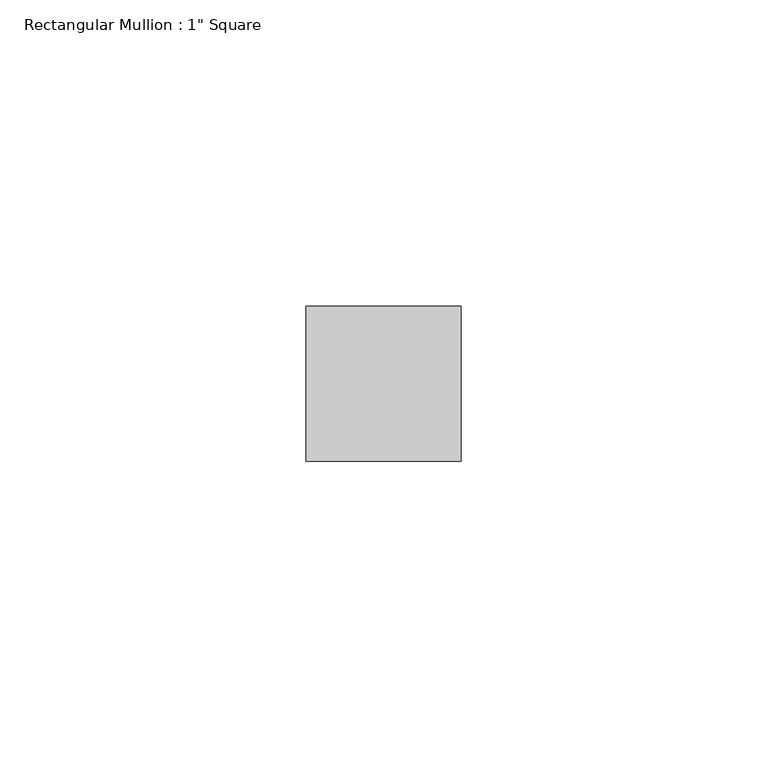
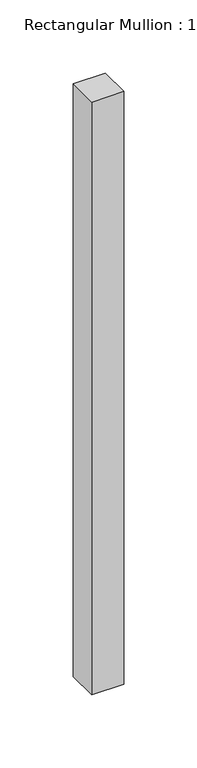
"""IFC4 building model written with IfcOpenShell, lengths in millimetres: member geometry."""

from ifc_helpers import new_model, si_unit, frame, origin, place, context, project, spatial, polyline, outline, extrude, source, transform, mapped, element, save


def member_84e80635(model_context):
    return source(origin(), model_context, "Body", "SweptSolid", [
        extrude(outline(polyline([(0.0, 12.7), (0.0, -12.7), (-25.4, -12.7), (-25.4, 12.7), (0.0, 12.7)])), frame((0.0, 0.0, -495.6398623), z_axis=(0.0, 0.0, 1.0), x_axis=(1.0, 0.0, 0.0)), (0.0, 0.0, 1.0), 495.6398623),
    ])


if __name__ == "__main__":
    model = new_model("IFC4")
    model_context = context("Model", 3, world=origin())
    ifc_project = project(units=[si_unit("LENGTHUNIT", "METRE", prefix="MILLI")], contexts=[model_context])
    site = spatial("IfcSite", under=ifc_project)
    building = spatial("IfcBuilding", under=site)
    placement = place(None, origin())
    member_shape = member_84e80635(model_context)
    element("IfcMember", 1, ObjectType="Rectangular Mullion : 1\" Square", at=placement, inside=building, context=model_context, shape_type="MappedRepresentation", body=[
        mapped(member_shape, transform((0.0, 0.0, 0.0), x_axis=(1.0, 0.0, 0.0), y_axis=(0.0, 1.0, 0.0), z_axis=(0.0, 0.0, 1.0))),
    ])
    save(model, "model.ifc")

# Revit data of these elements
# Type "Rectangular Mullion : 1\" Square"
#   built-in parameter 1007304 = 0.0833333 (stored number, unit not read)
#   built-in parameter 1007301 = 0.0416667 (stored number, unit not read)
#   built-in parameter 1007300 = 0.0416667 (stored number, unit not read)
